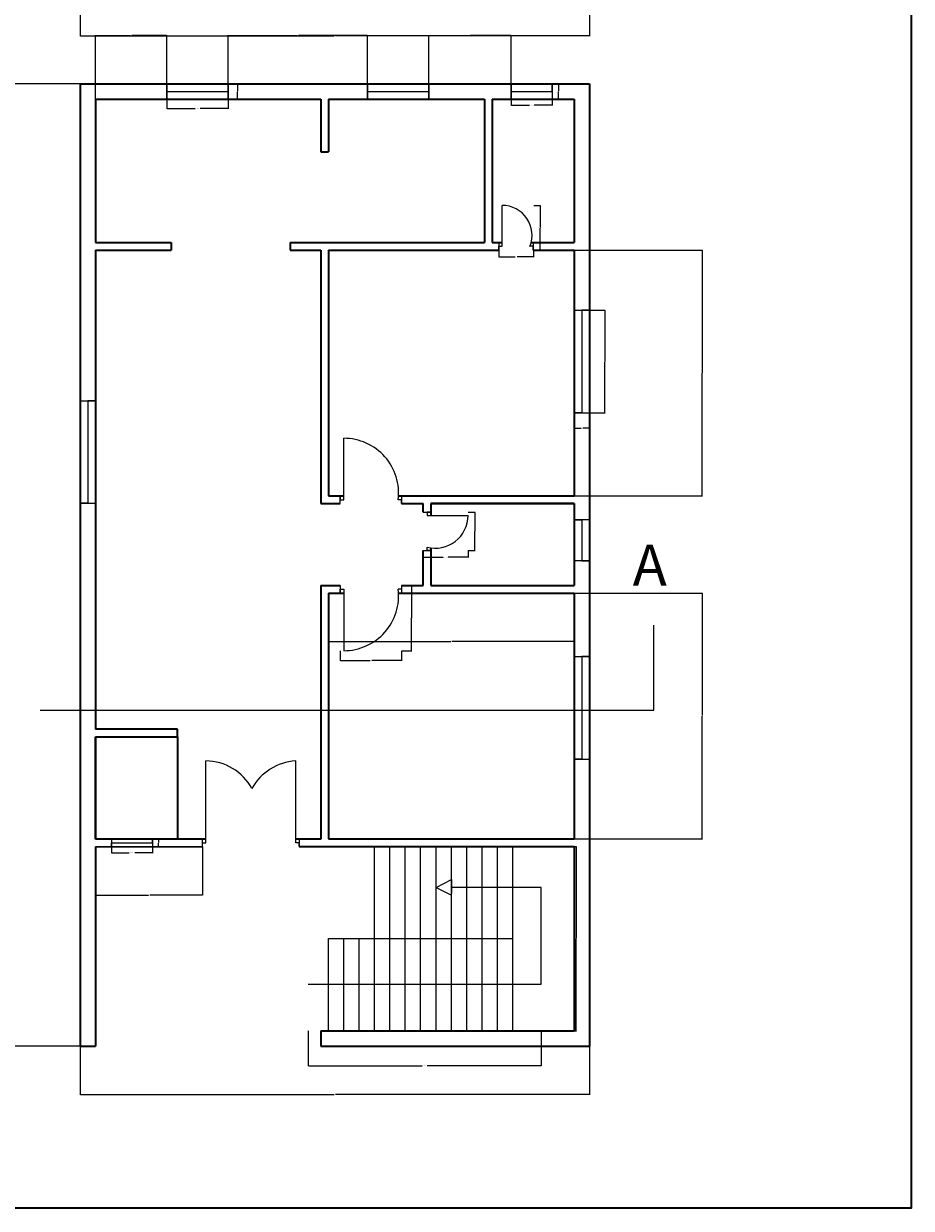
# Model space of a CAD drawing. Units: inches. Extents: x 2416 to 3391, y 1375 to 2496.
# Tile 3 of 13: x 2871 to 3391, y 1375 to 2069. Entities that reach past the tile are written whole.
import ezdxf

# ---------------------------------------------------------------- set-up
doc = ezdxf.new("R2010")
doc.units = ezdxf.units.IN
for name, color, linetype, lineweight in [('A-ANNO-DIMS', 2, 'Continuous', 18), ('A-ANNO-SYMB', 2, 'Continuous', 25), ('A-ANNO-TTLB', 7, 'Continuous', 35), ('A-DOOR', 3, 'Continuous', 20), ('A-FLOR-STRS', 7, 'Continuous', 20), ('A-GLAZ', 4, 'Continuous', 18), ('A-WALL', 7, 'Continuous', 35)]:
    doc.layers.add(name, color=color, linetype=linetype, lineweight=lineweight)
doc.styles.get("Standard").update_dxf_attribs({"font": 'arial.ttf'})
doc.dimstyles.get("Standard").update_dxf_attribs({"dimtxt": 0.18, "dimasz": 0.18, "dimexe": 0.18, "dimexo": 0.0625, "dimgap": 0.09, "dimtad": 0, "dimtih": 1, "dimtoh": 1, "dimdec": 4, "dimzin": 0, "dimdsep": 46, "dimtxsty": 'Standard', "dimcen": 0.09, "dimadec": 0, "dimazin": 0, "dimtfac": 1, "dimtdec": 4, "dimtofl": 0, "dimtmove": 0, "dimatfit": 3, "dimfxl": 1, "dimtolj": 1, "dimtzin": 0, "dimarcsym": 0})

# ---------------------------------------------------------------- blocks, each defined once
blk = doc.blocks.new('WINDOW-60IN')
for p, q in [((0, 60), (9, 60)), ((9, 60), (4.5, 60)), ((4.5, 60), (4.5, 0)), ((4.5, 0), (0, 0)), ((0, 0), (9, 0))]:
    blk.add_line(p, q)
blk = doc.blocks.new('WINDOW-36IN')
for p, q in [((0, 9), (0, 0)), ((36, 4.5), (36, 9)), ((36, 9), (36, 0)), ((0, 0), (0, 4.5)), ((0, 4.5), (36, 4.5))]:
    blk.add_line(p, q)
blk = doc.blocks.new('WINDOW-24IN')
for p, q in [((0, 9), (0, 0)), ((24, 4.5), (24, 9)), ((24, 9), (24, 0)), ((0, 0), (0, 4.5)), ((0, 4.5), (24, 4.5))]:
    blk.add_line(p, q)
blk = doc.blocks.new('WINDOW-24IN-INT')
for p, q in [((0, 4.49), (0.01, 0)), ((0.01, 0), (0, 2.24)), ((0, 2.24), (24, 2.24)), ((24, 2.24), (24, 4.49)), ((24, 4.49), (24.01, 0.03))]:
    blk.add_line(p, q)
blk = doc.blocks.new('DOOR-WC-NORTH')
for p, q in [((0, 0), (0, 24)), ((-2, 2.25), (-2, -2.25)), ((18.23, 2.25), (18.23, -2.25)), ((-2, -2.25), (-2, 0)), ((-2, 0), (0, 0)), ((18.23, 0), (16.23, 0)), ((18.23, -2.25), (18.23, 0))]:
    blk.add_line(p, q)
blk.add_arc((0, 6.51), 17.49, 338.1246, 90)
blk = doc.blocks.new('DOOR-BED-NORTH')
for p, q in [((0, 0), (0, 36)), ((-2, -2.25), (-2, 2.25)), ((-2, 2.25), (-2, 0)), ((33.94, 2.25), (33.94, -2.25)), ((-2, 0), (0, 0)), ((33.94, 0), (31.94, 0)), ((33.94, -2.25), (33.94, 0))]:
    blk.add_line(p, q)
blk.add_arc((0, 3.83), 32.17, 353.16573, 90)
blk = doc.blocks.new('DOOR-BED-SOUTH')
for p, q in [((-2, 2.25), (-2, -2.25)), ((33.94, 2.25), (33.94, -2.25)), ((-2, -2.25), (-2, 0)), ((-2, 0), (0, 0)), ((0, 0), (0, -36)), ((33.94, 0), (31.94, 0))]:
    blk.add_line(p, q)
blk.add_arc((0, -3.83), 32.17, 270, 6.83427)
blk = doc.blocks.new('DOOR-WC-SOUTH')
for p, q in [((-2.25, 2), (2.25, 2)), ((2.25, 2), (0, 2)), ((0, 2), (0, 0)), ((0, 0), (24, 0)), ((-2.25, -20.51), (2.25, -20.51)), ((0, -20.51), (0, -18.51)), ((2.25, -20.51), (0, -20.51))]:
    blk.add_line(p, q)
blk.add_arc((4.87, 0), 19.13, 255.26865, 0)
blk = doc.blocks.new('DOOR-ENTRY-PAIR')
for p, q in [((0, 0), (0, 48)), ((52.72, 0.04), (52.72, 48.04)), ((-2, 2.21), (-2, -2.21)), ((-2, 0), (0, 0)), ((54.72, 0.04), (52.72, 0.04)), ((54.72, 2.21), (54.73, -2.13)), ((54.73, -2.13), (54.72, 0.04))]:
    blk.add_line(p, q)
for centre, radius, start, end in [((0, 17.33), 30.67, 28.12018, 90), ((54.61, 16.65), 31.45, 93.43737, 151.22494)]:
    blk.add_arc(centre, radius, start, end)
blk = doc.blocks.new('STAIR-RETURN-PLAN')
for p, q in [((27, 0), (27, 108)), ((36, 0), (36, 108)), ((45, 0), (45, 108)), ((54, 0), (54, 108)), ((63, 0), (63, 108)), ((72, 0), (72, 108)), ((81, 0), (81, 108)), ((90, 0), (90, 108)), ((99, 0), (99, 108)), ((108, 0), (108, 108)), ((63, 83.93), (72, 88.71)), ((63, 83.93), (72, 79.53)), ((72, 88.71), (72, 80.54)), ((124.59, 83.93), (72, 83.93)), ((124.59, 27.37), (124.59, 83.93)), ((0, 0), (0, 54)), ((0, 54), (108, 54)), ((9, 0), (9, 54)), ((18, 0), (18, 54)), ((-11.89, 27.37), (124.59, 27.37)), ((-4.5, 0), (0, 0))]:
    blk.add_line(p, q)
blk = doc.blocks.new('*D17')
at = {"layer": 'A-ANNO-DIMS', "color": 0, "lineweight": -2, "transparency": 16777216}
for p, q in [((3202.75, 1901.41), (3211.87, 1901.41)), ((3211.69, 1901.23), (3211.69, 1871.59)), ((3211.69, 1841.59), (3211.69, 1871.23)), ((3202.75, 1841.41), (3211.87, 1841.41))]:
    blk.add_line(p, q, dxfattribs=at)
at = {"layer": 'A-ANNO-DIMS', "color": 0, "transparency": 16777216}
for points in [[(3211.66, 1901.23), (3211.72, 1901.23), (3211.69, 1901.41)], [(3211.66, 1841.59), (3211.72, 1841.59), (3211.69, 1841.41)]]:
    blk.add_solid(points, dxfattribs=at)
at = {"layer": 'Defpoints', "color": 0, "transparency": 16777216}
for p in [(3202.69, 1901.41), (3211.69, 1901.41), (3202.69, 1841.41)]:
    blk.add_point(p, dxfattribs=at)
at = {"layer": 'A-ANNO-DIMS', "color": 0, "transparency": 16777216, "insert": (3211.69, 1871.41), "char_height": 0.18, "attachment_point": 5}
blk.add_mtext('\\A1;SIDE WINDOW 60 TYP.', dxfattribs=at)
blk = doc.blocks.new('*D18')
at = {"layer": 'A-ANNO-DIMS', "color": 0, "lineweight": -2, "transparency": 16777216}
for p, q in [((3193.69, 1841.35), (3193.69, 1832.23)), ((3202.69, 1841.35), (3202.69, 1832.23)), ((3193.87, 1832.41), (3197.73, 1832.41)), ((3202.51, 1832.41), (3198.65, 1832.41))]:
    blk.add_line(p, q, dxfattribs=at)
at = {"layer": 'A-ANNO-DIMS', "color": 0, "transparency": 16777216}
for points in [[(3193.87, 1832.44), (3193.87, 1832.38), (3193.69, 1832.41)], [(3202.51, 1832.44), (3202.51, 1832.38), (3202.69, 1832.41)]]:
    blk.add_solid(points, dxfattribs=at)
at = {"layer": 'Defpoints', "color": 0, "transparency": 16777216}
for p in [(3193.69, 1841.41), (3202.69, 1841.41), (3202.69, 1832.41)]:
    blk.add_point(p, dxfattribs=at)
at = {"layer": 'A-ANNO-DIMS', "color": 0, "transparency": 16777216, "insert": (3198.19, 1832.41), "char_height": 0.18, "attachment_point": 5}
blk.add_mtext('\\A1;9 TYP.', dxfattribs=at)
blk = doc.blocks.new('*D19')
at = {"layer": 'A-ANNO-DIMS', "color": 0, "lineweight": -2, "transparency": 16777216}
for p, q in [((2954.98, 2025.11), (2954.98, 2019.59)), ((2990.98, 2025.11), (2990.98, 2019.59)), ((2955.16, 2019.77), (2971.49, 2019.77)), ((2990.8, 2019.77), (2974.48, 2019.77))]:
    blk.add_line(p, q, dxfattribs=at)
at = {"layer": 'A-ANNO-DIMS', "color": 0, "transparency": 16777216}
for points in [[(2955.16, 2019.8), (2955.16, 2019.74), (2954.98, 2019.77)], [(2990.8, 2019.8), (2990.8, 2019.74), (2990.98, 2019.77)]]:
    blk.add_solid(points, dxfattribs=at)
at = {"layer": 'Defpoints', "color": 0, "transparency": 16777216}
for p in [(2954.98, 2025.17), (2990.98, 2025.17), (2990.98, 2019.77)]:
    blk.add_point(p, dxfattribs=at)
at = {"layer": 'A-ANNO-DIMS', "color": 0, "transparency": 16777216, "insert": (2972.98, 2019.77), "char_height": 0.18, "attachment_point": 5}
blk.add_mtext('\\A1;REAR WINDOW 36 TYP.', dxfattribs=at)
blk = doc.blocks.new('*D20')
at = {"layer": 'A-ANNO-DIMS', "color": 0, "lineweight": -2, "transparency": 16777216}
for p, q in [((2991.04, 2034.17), (2996.56, 2034.17)), ((2996.38, 2033.99), (2996.38, 2029.85)), ((2996.38, 2025.35), (2996.38, 2029.49)), ((2991.04, 2025.17), (2996.56, 2025.17))]:
    blk.add_line(p, q, dxfattribs=at)
at = {"layer": 'A-ANNO-DIMS', "color": 0, "transparency": 16777216}
for points in [[(2996.35, 2033.99), (2996.41, 2033.99), (2996.38, 2034.17)], [(2996.35, 2025.35), (2996.41, 2025.35), (2996.38, 2025.17)]]:
    blk.add_solid(points, dxfattribs=at)
at = {"layer": 'Defpoints', "color": 0, "transparency": 16777216}
for p in [(2990.98, 2034.17), (2996.38, 2034.17), (2990.98, 2025.17)]:
    blk.add_point(p, dxfattribs=at)
at = {"layer": 'A-ANNO-DIMS', "color": 0, "transparency": 16777216, "insert": (2996.38, 2029.67), "char_height": 0.18, "attachment_point": 5}
blk.add_mtext('\\A1;9 TYP.', dxfattribs=at)
blk = doc.blocks.new('*D21')
at = {"layer": 'A-ANNO-DIMS', "color": 0, "lineweight": -2, "transparency": 16777216}
for p, q in [((3156.77, 2025.11), (3156.77, 2021.39)), ((3156.95, 2021.57), (3167.4, 2021.57)), ((3180.59, 2021.57), (3170.13, 2021.57)), ((3180.77, 2025.11), (3180.77, 2021.39))]:
    blk.add_line(p, q, dxfattribs=at)
at = {"layer": 'A-ANNO-DIMS', "color": 0, "transparency": 16777216}
for points in [[(3156.95, 2021.6), (3156.95, 2021.54), (3156.77, 2021.57)], [(3180.59, 2021.6), (3180.59, 2021.54), (3180.77, 2021.57)]]:
    blk.add_solid(points, dxfattribs=at)
at = {"layer": 'Defpoints', "color": 0, "transparency": 16777216}
for p in [(3156.77, 2025.17), (3180.77, 2025.17), (3180.77, 2021.57)]:
    blk.add_point(p, dxfattribs=at)
at = {"layer": 'A-ANNO-DIMS', "color": 0, "transparency": 16777216, "insert": (3168.77, 2021.57), "char_height": 0.18, "attachment_point": 5}
blk.add_mtext('\\A1;WC WINDOW 24 TYP.', dxfattribs=at)
blk = doc.blocks.new('*D22')
at = {"layer": 'A-ANNO-DIMS', "color": 0, "lineweight": -2, "transparency": 16777216}
for p, q in [((3180.83, 2034.17), (3184.55, 2034.17)), ((3184.37, 2033.99), (3184.37, 2029.85)), ((3184.37, 2025.35), (3184.37, 2029.49)), ((3180.83, 2025.17), (3184.55, 2025.17))]:
    blk.add_line(p, q, dxfattribs=at)
at = {"layer": 'A-ANNO-DIMS', "color": 0, "transparency": 16777216}
for points in [[(3184.34, 2033.99), (3184.4, 2033.99), (3184.37, 2034.17)], [(3184.34, 2025.35), (3184.4, 2025.35), (3184.37, 2025.17)]]:
    blk.add_solid(points, dxfattribs=at)
at = {"layer": 'Defpoints', "color": 0, "transparency": 16777216}
for p in [(3180.77, 2034.17), (3184.37, 2034.17), (3180.77, 2025.17)]:
    blk.add_point(p, dxfattribs=at)
at = {"layer": 'A-ANNO-DIMS', "color": 0, "transparency": 16777216, "insert": (3184.37, 2029.67), "char_height": 0.18, "attachment_point": 5}
blk.add_mtext('\\A1;9 TYP.', dxfattribs=at)
blk = doc.blocks.new('*D23')
at = {"layer": 'A-ANNO-DIMS', "color": 0, "lineweight": -2, "transparency": 16777216}
for p, q in [((2922.56, 1586.94), (2922.56, 1583.22)), ((2922.74, 1583.4), (2932.97, 1583.4)), ((2946.39, 1583.4), (2936.17, 1583.4)), ((2946.57, 1586.94), (2946.57, 1583.22))]:
    blk.add_line(p, q, dxfattribs=at)
at = {"layer": 'A-ANNO-DIMS', "color": 0, "transparency": 16777216}
for points in [[(2922.74, 1583.43), (2922.74, 1583.37), (2922.56, 1583.4)], [(2946.39, 1583.43), (2946.39, 1583.37), (2946.57, 1583.4)]]:
    blk.add_solid(points, dxfattribs=at)
at = {"layer": 'Defpoints', "color": 0, "transparency": 16777216}
for p in [(2922.56, 1587), (2946.57, 1587), (2946.57, 1583.4)]:
    blk.add_point(p, dxfattribs=at)
at = {"layer": 'A-ANNO-DIMS', "color": 0, "transparency": 16777216, "insert": (2934.57, 1583.4), "char_height": 0.18, "attachment_point": 5}
blk.add_mtext('\\A1;PORCH WINDOW 24 TYP.', dxfattribs=at)
blk = doc.blocks.new('*D24')
at = {"layer": 'A-ANNO-DIMS', "color": 0, "lineweight": -2, "transparency": 16777216}
for p, q in [((2946.63, 1591.49), (2950.35, 1591.49)), ((2950.17, 1591.31), (2950.17, 1589.43)), ((2946.63, 1587), (2950.35, 1587)), ((2950.17, 1587.18), (2950.17, 1589.07))]:
    blk.add_line(p, q, dxfattribs=at)
at = {"layer": 'A-ANNO-DIMS', "color": 0, "transparency": 16777216}
for points in [[(2950.14, 1591.31), (2950.2, 1591.31), (2950.17, 1591.49)], [(2950.14, 1587.18), (2950.2, 1587.18), (2950.17, 1587)]]:
    blk.add_solid(points, dxfattribs=at)
at = {"layer": 'Defpoints', "color": 0, "transparency": 16777216}
for p in [(2946.57, 1591.49), (2950.17, 1591.49), (2946.57, 1587)]:
    blk.add_point(p, dxfattribs=at)
at = {"layer": 'A-ANNO-DIMS', "color": 0, "transparency": 16777216, "insert": (2950.17, 1589.25), "char_height": 0.18, "attachment_point": 5}
blk.add_mtext('\\A1;4 TYP.', dxfattribs=at)
blk = doc.blocks.new('*D27')
at = {"layer": 'A-ANNO-DIMS', "color": 0, "lineweight": -2, "transparency": 16777216}
for p, q in [((3169.92, 1962.92), (3173.97, 1962.92)), ((3173.79, 1962.74), (3173.79, 1949.98)), ((3173.79, 1936.85), (3173.79, 1949.61)), ((3169.92, 1936.67), (3173.97, 1936.67))]:
    blk.add_line(p, q, dxfattribs=at)
at = {"layer": 'A-ANNO-DIMS', "color": 0, "transparency": 16777216}
for points in [[(3173.76, 1962.74), (3173.82, 1962.74), (3173.79, 1962.92)], [(3173.76, 1936.85), (3173.82, 1936.85), (3173.79, 1936.67)]]:
    blk.add_solid(points, dxfattribs=at)
at = {"layer": 'Defpoints', "color": 0, "transparency": 16777216}
for p in [(3169.86, 1962.92), (3173.79, 1962.92), (3169.86, 1936.67)]:
    blk.add_point(p, dxfattribs=at)
at = {"layer": 'A-ANNO-DIMS', "color": 0, "transparency": 16777216, "insert": (3173.79, 1949.8), "char_height": 0.18, "attachment_point": 5}
blk.add_mtext('\\A1;REAR WC DOOR 26 TYP.', dxfattribs=at)
blk = doc.blocks.new('*D28')
at = {"layer": 'A-ANNO-DIMS', "color": 0, "lineweight": -2, "transparency": 16777216}
for p, q in [((3149.47, 1936.61), (3149.47, 1932.55)), ((3149.65, 1932.73), (3159.13, 1932.73)), ((3169.68, 1932.73), (3160.19, 1932.73)), ((3169.86, 1936.61), (3169.86, 1932.55))]:
    blk.add_line(p, q, dxfattribs=at)
at = {"layer": 'A-ANNO-DIMS', "color": 0, "transparency": 16777216}
for points in [[(3149.65, 1932.76), (3149.65, 1932.7), (3149.47, 1932.73)], [(3169.68, 1932.76), (3169.68, 1932.7), (3169.86, 1932.73)]]:
    blk.add_solid(points, dxfattribs=at)
at = {"layer": 'Defpoints', "color": 0, "transparency": 16777216}
for p in [(3149.47, 1936.67), (3169.86, 1936.67), (3169.86, 1932.73)]:
    blk.add_point(p, dxfattribs=at)
at = {"layer": 'A-ANNO-DIMS', "color": 0, "transparency": 16777216, "insert": (3159.66, 1932.73), "char_height": 0.18, "attachment_point": 5}
blk.add_mtext('\\A1;20 TYP.', dxfattribs=at)
blk = doc.blocks.new('*D29')
at = {"layer": 'A-ANNO-DIMS', "color": 0, "lineweight": -2, "transparency": 16777216}
for p, q in [((3105.19, 1760.57), (3105.19, 1756.51)), ((3105.37, 1756.69), (3116.79, 1756.69)), ((3131.26, 1756.69), (3119.85, 1756.69)), ((3131.44, 1760.57), (3131.44, 1756.51))]:
    blk.add_line(p, q, dxfattribs=at)
at = {"layer": 'A-ANNO-DIMS', "color": 0, "transparency": 16777216}
for points in [[(3105.37, 1756.72), (3105.37, 1756.66), (3105.19, 1756.69)], [(3131.26, 1756.72), (3131.26, 1756.66), (3131.44, 1756.69)]]:
    blk.add_solid(points, dxfattribs=at)
at = {"layer": 'Defpoints', "color": 0, "transparency": 16777216}
for p in [(3105.19, 1760.63), (3131.44, 1760.63), (3131.44, 1756.69)]:
    blk.add_point(p, dxfattribs=at)
at = {"layer": 'A-ANNO-DIMS', "color": 0, "transparency": 16777216, "insert": (3118.32, 1756.69), "char_height": 0.18, "attachment_point": 5}
blk.add_mtext('\\A1;HALL WC DOOR 26 TYP.', dxfattribs=at)
blk = doc.blocks.new('*D30')
at = {"layer": 'A-ANNO-DIMS', "color": 0, "lineweight": -2, "transparency": 16777216}
for p, q in [((3131.5, 1783.13), (3135.56, 1783.13)), ((3135.38, 1782.95), (3135.38, 1772.06)), ((3135.38, 1760.81), (3135.38, 1771.7)), ((3131.5, 1760.63), (3135.56, 1760.63))]:
    blk.add_line(p, q, dxfattribs=at)
at = {"layer": 'A-ANNO-DIMS', "color": 0, "transparency": 16777216}
for points in [[(3135.35, 1782.95), (3135.41, 1782.95), (3135.38, 1783.13)], [(3135.35, 1760.81), (3135.41, 1760.81), (3135.38, 1760.63)]]:
    blk.add_solid(points, dxfattribs=at)
at = {"layer": 'Defpoints', "color": 0, "transparency": 16777216}
for p in [(3131.44, 1783.13), (3135.38, 1783.13), (3131.44, 1760.63)]:
    blk.add_point(p, dxfattribs=at)
at = {"layer": 'A-ANNO-DIMS', "color": 0, "transparency": 16777216, "insert": (3135.38, 1771.88), "char_height": 0.18, "attachment_point": 5}
blk.add_mtext('\\A1;23 TYP.', dxfattribs=at)
blk = doc.blocks.new('*D33')
at = {"layer": 'A-ANNO-DIMS', "color": 0, "lineweight": -2, "transparency": 16777216}
for p, q in [((3092.63, 1740.17), (3098.48, 1740.17)), ((3098.3, 1739.99), (3098.3, 1721.23)), ((3098.3, 1702.1), (3098.3, 1720.86)), ((3092.63, 1701.92), (3098.48, 1701.92))]:
    blk.add_line(p, q, dxfattribs=at)
at = {"layer": 'A-ANNO-DIMS', "color": 0, "transparency": 16777216}
for points in [[(3098.27, 1739.99), (3098.33, 1739.99), (3098.3, 1740.17)], [(3098.27, 1702.1), (3098.33, 1702.1), (3098.3, 1701.92)]]:
    blk.add_solid(points, dxfattribs=at)
at = {"layer": 'Defpoints', "color": 0, "transparency": 16777216}
for p in [(3092.56, 1740.17), (3098.3, 1740.17), (3092.56, 1701.92)]:
    blk.add_point(p, dxfattribs=at)
at = {"layer": 'A-ANNO-DIMS', "color": 0, "transparency": 16777216, "insert": (3098.3, 1721.05), "char_height": 0.18, "attachment_point": 5}
blk.add_mtext('\\A1;BEDROOM 1 DOOR 38 TYP.', dxfattribs=at)
blk = doc.blocks.new('*D34')
at = {"layer": 'A-ANNO-DIMS', "color": 0, "lineweight": -2, "transparency": 16777216}
for p, q in [((3056.62, 1701.86), (3056.62, 1696)), ((3092.56, 1701.86), (3092.56, 1696)), ((3056.8, 1696.18), (3074.06, 1696.18)), ((3092.38, 1696.18), (3075.12, 1696.18))]:
    blk.add_line(p, q, dxfattribs=at)
at = {"layer": 'A-ANNO-DIMS', "color": 0, "transparency": 16777216}
for points in [[(3056.8, 1696.21), (3056.8, 1696.15), (3056.62, 1696.18)], [(3092.38, 1696.21), (3092.38, 1696.15), (3092.56, 1696.18)]]:
    blk.add_solid(points, dxfattribs=at)
at = {"layer": 'Defpoints', "color": 0, "transparency": 16777216}
for p in [(3056.62, 1701.92), (3092.56, 1701.92), (3092.56, 1696.18)]:
    blk.add_point(p, dxfattribs=at)
at = {"layer": 'A-ANNO-DIMS', "color": 0, "transparency": 16777216, "insert": (3074.59, 1696.18), "char_height": 0.18, "attachment_point": 5}
blk.add_mtext('\\A1;36 TYP.', dxfattribs=at)
blk = doc.blocks.new('*D37')
at = {"layer": 'A-ANNO-DIMS', "color": 0, "lineweight": -2, "transparency": 16777216}
for p, q in [((3037.8, 1479.11), (3037.8, 1458.52)), ((3174.28, 1479.11), (3174.28, 1458.52)), ((3037.98, 1458.7), (3104.49, 1458.7)), ((3174.1, 1458.7), (3107.6, 1458.7))]:
    blk.add_line(p, q, dxfattribs=at)
at = {"layer": 'A-ANNO-DIMS', "color": 0, "transparency": 16777216}
for points in [[(3037.98, 1458.73), (3037.98, 1458.67), (3037.8, 1458.7)], [(3174.1, 1458.73), (3174.1, 1458.67), (3174.28, 1458.7)]]:
    blk.add_solid(points, dxfattribs=at)
at = {"layer": 'Defpoints', "color": 0, "transparency": 16777216}
for p in [(3037.8, 1479.17), (3174.28, 1479.17), (3174.28, 1458.7)]:
    blk.add_point(p, dxfattribs=at)
at = {"layer": 'A-ANNO-DIMS', "color": 0, "transparency": 16777216, "insert": (3106.04, 1458.7), "char_height": 0.18, "attachment_point": 5}
blk.add_mtext('\\A1;RETURN STAIR 136 TYP.', dxfattribs=at)
blk = doc.blocks.new('*D38')
at = {"layer": 'A-ANNO-DIMS', "color": 0, "lineweight": -2, "transparency": 16777216}
for p, q in [((3174.35, 1587.17), (3194.93, 1587.17)), ((3194.75, 1586.99), (3194.75, 1533.35)), ((3194.75, 1479.35), (3194.75, 1532.99)), ((3174.35, 1479.17), (3194.93, 1479.17))]:
    blk.add_line(p, q, dxfattribs=at)
at = {"layer": 'A-ANNO-DIMS', "color": 0, "transparency": 16777216}
for points in [[(3194.72, 1586.99), (3194.78, 1586.99), (3194.75, 1587.17)], [(3194.72, 1479.35), (3194.78, 1479.35), (3194.75, 1479.17)]]:
    blk.add_solid(points, dxfattribs=at)
at = {"layer": 'Defpoints', "color": 0, "transparency": 16777216}
for p in [(3174.28, 1587.17), (3194.75, 1587.17), (3174.28, 1479.17)]:
    blk.add_point(p, dxfattribs=at)
at = {"layer": 'A-ANNO-DIMS', "color": 0, "transparency": 16777216, "insert": (3194.75, 1533.17), "char_height": 0.18, "attachment_point": 5}
blk.add_mtext('\\A1;108 TYP.', dxfattribs=at)
blk = doc.blocks.new('*D54')
at = {"layer": 'A-ANNO-DIMS', "color": 0, "lineweight": -2, "transparency": 16777216}
for p, q in [((2904.19, 1470.11), (2904.19, 1441.64)), ((3202.69, 1470.11), (3202.69, 1441.64)), ((2904.37, 1441.82), (3053.05, 1441.82)), ((3202.51, 1441.82), (3053.84, 1441.82))]:
    blk.add_line(p, q, dxfattribs=at)
at = {"layer": 'A-ANNO-DIMS', "color": 0, "transparency": 16777216}
for points in [[(2904.37, 1441.85), (2904.37, 1441.79), (2904.19, 1441.82)], [(3202.51, 1441.85), (3202.51, 1441.79), (3202.69, 1441.82)]]:
    blk.add_solid(points, dxfattribs=at)
at = {"layer": 'Defpoints', "color": 0, "transparency": 16777216}
for p in [(2904.19, 1470.17), (3202.69, 1470.17), (3202.69, 1441.82)]:
    blk.add_point(p, dxfattribs=at)
at = {"layer": 'A-ANNO-DIMS', "color": 0, "transparency": 16777216, "insert": (3053.44, 1441.82), "char_height": 0.18, "attachment_point": 5}
blk.add_mtext('\\A1;298.5', dxfattribs=at)
blk = doc.blocks.new('*D55')
at = {"layer": 'A-ANNO-DIMS', "color": 0, "lineweight": -2, "transparency": 16777216}
for p, q in [((2904.13, 2034.17), (2852.3, 2034.17)), ((2852.48, 2033.99), (2852.48, 1752.35)), ((2852.48, 1470.35), (2852.48, 1751.99)), ((2904.13, 1470.17), (2852.3, 1470.17))]:
    blk.add_line(p, q, dxfattribs=at)
at = {"layer": 'A-ANNO-DIMS', "color": 0, "transparency": 16777216}
for points in [[(2852.45, 2033.99), (2852.51, 2033.99), (2852.48, 2034.17)], [(2852.45, 1470.35), (2852.51, 1470.35), (2852.48, 1470.17)]]:
    blk.add_solid(points, dxfattribs=at)
at = {"layer": 'Defpoints', "color": 0, "transparency": 16777216}
for p in [(2852.48, 2034.17), (2904.19, 2034.17), (2904.19, 1470.17)]:
    blk.add_point(p, dxfattribs=at)
at = {"layer": 'A-ANNO-DIMS', "color": 0, "transparency": 16777216, "insert": (2852.48, 1752.17), "char_height": 0.18, "attachment_point": 5}
blk.add_mtext('\\A1;564', dxfattribs=at)
blk = doc.blocks.new('*D56')
at = {"layer": 'A-ANNO-DIMS', "color": 0, "lineweight": -2, "transparency": 16777216}
for p, q in [((2913.19, 2025.23), (2913.19, 2062.7)), ((2913.37, 2062.52), (2933.69, 2062.52)), ((2954.8, 2062.52), (2934.48, 2062.52)), ((2954.98, 2025.23), (2954.98, 2062.7))]:
    blk.add_line(p, q, dxfattribs=at)
at = {"layer": 'A-ANNO-DIMS', "color": 0, "transparency": 16777216}
for points in [[(2913.37, 2062.55), (2913.37, 2062.49), (2913.19, 2062.52)], [(2954.8, 2062.55), (2954.8, 2062.49), (2954.98, 2062.52)]]:
    blk.add_solid(points, dxfattribs=at)
at = {"layer": 'Defpoints', "color": 0, "transparency": 16777216}
for p in [(2954.98, 2062.52), (2913.19, 2025.17), (2954.98, 2025.17)]:
    blk.add_point(p, dxfattribs=at)
at = {"layer": 'A-ANNO-DIMS', "color": 0, "transparency": 16777216, "insert": (2934.09, 2062.52), "char_height": 0.18, "attachment_point": 5}
blk.add_mtext('\\A1;41.79', dxfattribs=at)
blk = doc.blocks.new('*D57')
at = {"layer": 'A-ANNO-DIMS', "color": 0, "lineweight": -2, "transparency": 16777216}
for p, q in [((2990.98, 2025.23), (2990.98, 2062.7)), ((2991.16, 2062.52), (3031.33, 2062.52)), ((3072.29, 2062.52), (3032.12, 2062.52)), ((3072.47, 2025.23), (3072.47, 2062.7))]:
    blk.add_line(p, q, dxfattribs=at)
at = {"layer": 'A-ANNO-DIMS', "color": 0, "transparency": 16777216}
for points in [[(2991.16, 2062.55), (2991.16, 2062.49), (2990.98, 2062.52)], [(3072.29, 2062.55), (3072.29, 2062.49), (3072.47, 2062.52)]]:
    blk.add_solid(points, dxfattribs=at)
at = {"layer": 'Defpoints', "color": 0, "transparency": 16777216}
for p in [(3072.47, 2062.52), (2990.98, 2025.17), (3072.47, 2025.17)]:
    blk.add_point(p, dxfattribs=at)
at = {"layer": 'A-ANNO-DIMS', "color": 0, "transparency": 16777216, "insert": (3031.72, 2062.52), "char_height": 0.18, "attachment_point": 5}
blk.add_mtext('\\A1;81.48', dxfattribs=at)
blk = doc.blocks.new('*D58')
at = {"layer": 'A-ANNO-DIMS', "color": 0, "lineweight": -2, "transparency": 16777216}
for p, q in [((3108.47, 2025.23), (3108.47, 2062.7)), ((3108.65, 2062.52), (3132.29, 2062.52)), ((3156.59, 2062.52), (3132.94, 2062.52)), ((3156.77, 2025.23), (3156.77, 2062.7))]:
    blk.add_line(p, q, dxfattribs=at)
at = {"layer": 'A-ANNO-DIMS', "color": 0, "transparency": 16777216}
for points in [[(3108.65, 2062.55), (3108.65, 2062.49), (3108.47, 2062.52)], [(3156.59, 2062.55), (3156.59, 2062.49), (3156.77, 2062.52)]]:
    blk.add_solid(points, dxfattribs=at)
at = {"layer": 'Defpoints', "color": 0, "transparency": 16777216}
for p in [(3156.77, 2062.52), (3108.47, 2025.17), (3156.77, 2025.17)]:
    blk.add_point(p, dxfattribs=at)
at = {"layer": 'A-ANNO-DIMS', "color": 0, "transparency": 16777216, "insert": (3132.62, 2062.52), "char_height": 0.18, "attachment_point": 5}
blk.add_mtext('\\A1;48.3', dxfattribs=at)
blk = doc.blocks.new('*D59')
at = {"layer": 'A-ANNO-DIMS', "color": 0, "lineweight": -2, "transparency": 16777216}
for p, q in [((3049.69, 1735.61), (3049.69, 1707.14)), ((3193.69, 1735.61), (3193.69, 1707.14)), ((3049.87, 1707.32), (3121.41, 1707.32)), ((3193.51, 1707.32), (3121.97, 1707.32))]:
    blk.add_line(p, q, dxfattribs=at)
at = {"layer": 'A-ANNO-DIMS', "color": 0, "transparency": 16777216}
for points in [[(3049.87, 1707.35), (3049.87, 1707.29), (3049.69, 1707.32)], [(3193.51, 1707.35), (3193.51, 1707.29), (3193.69, 1707.32)]]:
    blk.add_solid(points, dxfattribs=at)
at = {"layer": 'Defpoints', "color": 0, "transparency": 16777216}
for p in [(3049.69, 1735.67), (3193.69, 1735.67), (3049.69, 1707.32)]:
    blk.add_point(p, dxfattribs=at)
at = {"layer": 'A-ANNO-DIMS', "color": 0, "transparency": 16777216, "insert": (3121.69, 1707.32), "char_height": 0.18, "attachment_point": 5}
blk.add_mtext('\\A1;144', dxfattribs=at)
blk = doc.blocks.new('*D60')
at = {"layer": 'A-ANNO-DIMS', "color": 0, "lineweight": -2, "transparency": 16777216}
for p, q in [((3193.75, 1936.67), (3268.85, 1936.67)), ((3268.67, 1936.49), (3268.67, 1864.85)), ((3268.67, 1792.85), (3268.67, 1864.49)), ((3193.75, 1792.67), (3268.85, 1792.67))]:
    blk.add_line(p, q, dxfattribs=at)
at = {"layer": 'A-ANNO-DIMS', "color": 0, "transparency": 16777216}
for points in [[(3268.64, 1936.49), (3268.7, 1936.49), (3268.67, 1936.67)], [(3268.64, 1792.85), (3268.7, 1792.85), (3268.67, 1792.67)]]:
    blk.add_solid(points, dxfattribs=at)
at = {"layer": 'Defpoints', "color": 0, "transparency": 16777216}
for p in [(3193.69, 1936.67), (3268.67, 1936.67), (3193.69, 1792.67)]:
    blk.add_point(p, dxfattribs=at)
at = {"layer": 'A-ANNO-DIMS', "color": 0, "transparency": 16777216, "insert": (3268.67, 1864.67), "char_height": 0.18, "attachment_point": 5}
blk.add_mtext('\\A1;144', dxfattribs=at)
blk = doc.blocks.new('*D61')
at = {"layer": 'A-ANNO-DIMS', "color": 0, "lineweight": -2, "transparency": 16777216}
for p, q in [((3193.75, 1735.67), (3268.85, 1735.67)), ((3268.67, 1735.49), (3268.67, 1663.85)), ((3268.67, 1591.85), (3268.67, 1663.49)), ((3193.75, 1591.67), (3268.85, 1591.67))]:
    blk.add_line(p, q, dxfattribs=at)
at = {"layer": 'A-ANNO-DIMS', "color": 0, "transparency": 16777216}
for points in [[(3268.64, 1735.49), (3268.7, 1735.49), (3268.67, 1735.67)], [(3268.64, 1591.85), (3268.7, 1591.85), (3268.67, 1591.67)]]:
    blk.add_solid(points, dxfattribs=at)
at = {"layer": 'Defpoints', "color": 0, "transparency": 16777216}
for p in [(3193.69, 1735.67), (3268.67, 1735.67), (3193.69, 1591.67)]:
    blk.add_point(p, dxfattribs=at)
at = {"layer": 'A-ANNO-DIMS', "color": 0, "transparency": 16777216, "insert": (3268.67, 1663.67), "char_height": 0.18, "attachment_point": 5}
blk.add_mtext('\\A1;144', dxfattribs=at)
blk = doc.blocks.new('*D62')
at = {"layer": 'A-ANNO-DIMS', "color": 0, "lineweight": -2, "transparency": 16777216}
for p, q in [((2913.19, 1586.93), (2913.23, 1558.46)), ((2975.76, 1587.01), (2975.8, 1558.55)), ((2913.41, 1558.64), (2944.12, 1558.68)), ((2975.62, 1558.72), (2944.91, 1558.68))]:
    blk.add_line(p, q, dxfattribs=at)
at = {"layer": 'A-ANNO-DIMS', "color": 0, "transparency": 16777216}
for points in [[(2913.41, 1558.67), (2913.41, 1558.61), (2913.23, 1558.64)], [(2975.62, 1558.75), (2975.62, 1558.69), (2975.8, 1558.73)]]:
    blk.add_solid(points, dxfattribs=at)
at = {"layer": 'Defpoints', "color": 0, "transparency": 16777216}
for p in [(2913.19, 1586.99), (2975.76, 1587.08), (2913.23, 1558.64)]:
    blk.add_point(p, dxfattribs=at)
at = {"layer": 'A-ANNO-DIMS', "color": 0, "transparency": 16777216, "insert": (2944.51, 1558.68), "char_height": 0.18, "attachment_point": 5}
blk.add_mtext('\\A1;62.57', dxfattribs=at)
blk = doc.blocks.new('*D83')
at = {"layer": 'A-ANNO-DIMS', "color": 0, "lineweight": -2, "transparency": 16777216}
for p, q in [((2904.19, 2125.8), (2904.19, 2062.03)), ((3202.69, 2125.8), (3202.69, 2062.03)), ((2904.37, 2062.21), (3053.05, 2062.21)), ((3202.51, 2062.21), (3053.84, 2062.21))]:
    blk.add_line(p, q, dxfattribs=at)
at = {"layer": 'A-ANNO-DIMS', "color": 0, "transparency": 16777216}
for points in [[(2904.37, 2062.24), (2904.37, 2062.18), (2904.19, 2062.21)], [(3202.51, 2062.24), (3202.51, 2062.18), (3202.69, 2062.21)]]:
    blk.add_solid(points, dxfattribs=at)
at = {"layer": 'Defpoints', "color": 0, "transparency": 16777216}
for p in [(2904.19, 2125.86), (3202.69, 2125.86), (3202.69, 2062.21)]:
    blk.add_point(p, dxfattribs=at)
at = {"layer": 'A-ANNO-DIMS', "color": 0, "transparency": 16777216, "insert": (3053.44, 2062.21), "char_height": 0.18, "attachment_point": 5}
blk.add_mtext('\\A1;298.5', dxfattribs=at)

msp = doc.modelspace()

# ---------------------------------------------------------------- linework, layer by layer
at = {"layer": 'A-ANNO-SYMB'}
for p, q in [((3240.3152, 1666.9855), (3240.3152, 1716.9621)), ((2880.8281, 1666.9855), (3240.3152, 1666.9855))]:
    msp.add_line(p, q, dxfattribs=at)
at = {"layer": 'A-ANNO-TTLB'}
msp.add_lwpolyline([(2416.4678, 2496.0939), (3391.2022, 2496.0939), (3391.2022, 1375.1104), (2416.4678, 1375.1104)], close=True, dxfattribs=at)
at = {"layer": 'A-WALL'}
for p, q in [((2904.1924, 2034.17), (2904.1924, 1470.17)), ((2904.1924, 2034.17), (3202.6924, 2034.17)), ((3202.6924, 2034.17), (3202.6924, 1470.17)), ((2913.1924, 2025.17), (2913.1924, 1941.17)), ((2913.1924, 2025.17), (3045.1924, 2025.17)), ((3045.1924, 2025.17), (3045.1924, 1994.3212)), ((3049.6924, 2025.17), (3049.6924, 1994.3212)), ((3049.6924, 2025.17), (3141.1924, 2025.17)), ((3141.1924, 2025.17), (3141.1924, 1941.17)), ((3145.6924, 2025.17), (3145.6924, 1941.17)), ((3145.6924, 2025.17), (3193.6924, 2025.17)), ((3193.6924, 2025.17), (3193.6924, 1941.17)), ((3045.1924, 1994.3212), (3049.6924, 1994.3212)), ((2913.1924, 1941.17), (2957.5166, 1941.17)), ((2957.5166, 1941.17), (2957.5166, 1936.67)), ((3027.1924, 1941.17), (3141.1924, 1941.17)), ((3027.1924, 1941.17), (3027.1924, 1936.67)), ((3145.6924, 1941.17), (3151.4662, 1941.17)), ((3168.4233, 1941.17), (3193.6924, 1941.17)), ((2913.1924, 1936.67), (2913.1924, 1655.9896)), ((2913.1924, 1936.67), (2957.5166, 1936.67)), ((3027.1924, 1936.67), (3045.1924, 1936.67)), ((3045.1924, 1936.67), (3045.1924, 1788.17)), ((3049.6924, 1936.67), (3049.6924, 1792.67)), ((3049.6924, 1936.67), (3149.4662, 1936.67)), ((3169.6924, 1936.67), (3193.6924, 1936.67)), ((3193.6924, 1936.67), (3193.6924, 1792.67)), ((3049.6924, 1792.67), (3058.6195, 1792.67)), ((3090.7524, 1792.67), (3193.6924, 1792.67)), ((3045.1924, 1788.17), (3056.6195, 1788.17)), ((3092.5626, 1788.17), (3105.1924, 1788.17)), ((3105.1924, 1783.1345), (3105.1924, 1788.17)), ((3109.6924, 1788.17), (3193.6924, 1788.17)), ((3193.6924, 1788.17), (3109.6924, 1788.17)), ((3109.6924, 1788.17), (3109.6924, 1781.1345)), ((3193.6924, 1788.17), (3193.6924, 1740.17)), ((3105.1924, 1740.17), (3105.1924, 1760.6291)), ((3109.6924, 1762.1797), (3109.6924, 1740.17)), ((3045.1924, 1740.17), (3045.1924, 1591.4896)), ((3045.1924, 1740.17), (3056.6195, 1740.17)), ((3092.5626, 1740.17), (3105.1924, 1740.17)), ((3109.6924, 1740.17), (3193.6924, 1740.17)), ((3049.6924, 1735.67), (3049.6924, 1591.67)), ((3049.6924, 1735.67), (3058.6195, 1735.67)), ((3090.7524, 1735.67), (3193.6924, 1735.67)), ((3193.6924, 1735.67), (3193.6924, 1591.67)), ((2961.1924, 1655.9896), (2913.1924, 1655.9896)), ((2961.1924, 1651.4896), (2961.1924, 1655.9896)), ((2913.1924, 1651.4896), (2913.1924, 1591.4896)), ((2913.1924, 1591.4896), (2913.1924, 1651.4896)), ((2913.1924, 1651.4896), (2961.1924, 1651.4896)), ((2961.1924, 1651.4896), (2961.1924, 1591.4896)), ((2977.7552, 1591.4896), (2913.1924, 1591.4896)), ((3045.1924, 1591.4896), (3030.4791, 1591.4896)), ((3049.6924, 1591.67), (3193.6924, 1591.67)), ((2913.1924, 1586.9896), (2975.7582, 1587.0751)), ((2913.1924, 1586.9896), (2913.1924, 1470.17)), ((3032.482, 1587.1527), (3045.1924, 1587.17)), ((3045.1924, 1587.17), (3193.6924, 1587.17)), ((3193.6924, 1587.17), (3193.6924, 1479.17)), ((3045.1924, 1479.17), (3045.1924, 1470.17)), ((3045.1924, 1479.17), (3193.6924, 1479.17)), ((2904.1924, 1470.17), (2913.1924, 1470.17)), ((3045.1924, 1470.17), (3202.6924, 1470.17))]:
    msp.add_line(p, q, dxfattribs=at)

# ---------------------------------------------------------------- block references
at = {"layer": 'A-DOOR'}
for name, p in [('DOOR-WC-NORTH', (3151.4662, 1938.92)), ('DOOR-BED-NORTH', (3058.6195, 1790.42)), ('DOOR-WC-SOUTH', (3107.4424, 1781.1345)), ('DOOR-BED-SOUTH', (3058.6195, 1737.92)), ('DOOR-ENTRY-PAIR', (2977.7552, 1589.2824))]:
    msp.add_blockref(name, p, dxfattribs=at)
at = {"layer": 'A-FLOR-STRS'}
msp.add_blockref('STAIR-RETURN-PLAN', (3049.6924, 1479.17), dxfattribs=at)
at = {"layer": 'A-GLAZ'}
for name, p in [('WINDOW-36IN', (2954.9821, 2025.17)), ('WINDOW-36IN', (3072.4662, 2025.17)), ('WINDOW-24IN', (3156.7671, 2025.17)), ('WINDOW-60IN', (3193.6921, 1841.41)), ('WINDOW-60IN', (2904.1921, 1788.3842)), ('WINDOW-60IN', (3193.6921, 1638.4452)), ('WINDOW-24IN-INT', (2922.5621, 1587.002))]:
    msp.add_blockref(name, p, dxfattribs=at)
at = {"layer": 'A-GLAZ', "rotation": 270.0000000000002}
msp.add_blockref('WINDOW-24IN', (3193.6924, 1778.581), dxfattribs=at)

# ---------------------------------------------------------------- texts
at = {"layer": 'A-ANNO-SYMB', "insert": (3227.9919, 1764.1232), "char_height": 24, "attachment_point": 1}
msp.add_mtext_dynamic_manual_height_columns('A', width=43.659534, gutter_width=12.5, heights=[0], dxfattribs=at)

# ---------------------------------------------------------------- dimensions: what is measured, and where the dimension line sits
at = {"layer": 'A-ANNO-DIMS'}
for base, p1, p2, override, picture, middle in [((3202.6924, 2062.2125), (2904.1924, 2125.8608), (3202.6924, 2125.8608), {"dimdec": 1, "dimlfac": 1, "dimrnd": 0, "dimzin": 0, "dimdsep": 46, "dimlunit": 2}, '*D83', (3053.4424, 2062.2125)), ((2954.9819, 2062.52), (2913.1924, 2025.17), (2954.9819, 2025.17), {"dimdec": 2, "dimlfac": 1, "dimrnd": 0, "dimzin": 0, "dimdsep": 46, "dimlunit": 2}, '*D56', (2934.0872, 2062.52)), ((3072.4661, 2062.52), (2990.9819, 2025.17), (3072.4661, 2025.17), {"dimdec": 2, "dimlfac": 1, "dimrnd": 0, "dimzin": 0, "dimdsep": 46, "dimlunit": 2}, '*D57', (3031.724, 2062.52)), ((3156.7667, 2062.52), (3108.4661, 2025.17), (3156.7667, 2025.17), {"dimdec": 1, "dimlfac": 1, "dimrnd": 0, "dimzin": 0, "dimdsep": 46, "dimlunit": 2}, '*D58', (3132.6164, 2062.52)), ((3202.6924, 1441.82), (2904.1924, 1470.17), (3202.6924, 1470.17), {"dimdec": 1, "dimlfac": 1, "dimrnd": 0, "dimzin": 0, "dimdsep": 46, "dimlunit": 2}, '*D54', (3053.4424, 1441.82))]:
    dim = msp.add_linear_dim(base=base, p1=p1, p2=p2, dimstyle='Standard', override=override, dxfattribs=at)
    dim.commit()
    dim.dimension.update_dxf_attribs({"geometry": picture, "text_midpoint": middle})
for base, p1, p2, angle, override, picture, middle in [((2852.4781, 2034.17), (2904.1924, 1470.17), (2904.1924, 2034.17), 90, {"dimdec": 0, "dimlfac": 1, "dimrnd": 0, "dimzin": 0, "dimdsep": 46, "dimlunit": 2}, '*D55', (2852.4781, 1752.17)), ((3268.6652, 1936.67), (3193.6924, 1792.67), (3193.6924, 1936.67), 90, {"dimdec": 0, "dimlfac": 1, "dimrnd": 0, "dimzin": 0, "dimdsep": 46, "dimlunit": 2}, '*D60', (3268.6652, 1864.67)), ((3049.6924, 1707.32), (3193.6924, 1735.67), (3049.6924, 1735.67), 180, {"dimdec": 0, "dimlfac": 1, "dimrnd": 0, "dimzin": 0, "dimdsep": 46, "dimlunit": 2}, '*D59', (3121.6924, 1707.32)), ((3268.6652, 1735.67), (3193.6924, 1591.67), (3193.6924, 1735.67), 90, {"dimdec": 0, "dimlfac": 1, "dimrnd": 0, "dimzin": 0, "dimdsep": 46, "dimlunit": 2}, '*D61', (3268.6652, 1663.67)), ((2913.2312, 1558.6396), (2975.7582, 1587.0751), (2913.1924, 1586.9896), 180.0783088, {"dimdec": 2, "dimlfac": 1, "dimrnd": 0, "dimzin": 0, "dimdsep": 46, "dimlunit": 2}, '*D62', (2944.514, 1558.6824))]:
    dim = msp.add_linear_dim(base=base, p1=p1, p2=p2, angle=angle, dimstyle='Standard', override=override, dxfattribs=at)
    dim.commit()
    dim.dimension.update_dxf_attribs({"geometry": picture, "text_midpoint": middle})
for base, p1, p2, text, picture, middle in [((2996.3819, 2034.17), (2990.9819, 2025.17), (2990.9819, 2034.17), '<> TYP.', '*D20', (2996.3819, 2029.67)), ((3184.3667, 2034.17), (3180.7667, 2025.17), (3180.7667, 2034.17), '<> TYP.', '*D22', (3184.3667, 2029.67)), ((3173.7932, 1962.92), (3169.8557, 1936.67), (3169.8557, 1962.92), 'REAR WC DOOR <> TYP.', '*D27', (3173.7932, 1949.795)), ((3211.6924, 1901.4103), (3202.6924, 1841.4103), (3202.6924, 1901.4103), 'SIDE WINDOW <> TYP.', '*D17', (3211.6924, 1871.4103)), ((3135.3799, 1783.1345), (3131.4424, 1760.6291), (3131.4424, 1783.1345), '<> TYP.', '*D30', (3135.3799, 1771.8818)), ((3098.3001, 1740.17), (3092.5626, 1701.92), (3092.5626, 1740.17), 'BEDROOM 1 DOOR <> TYP.', '*D33', (3098.3001, 1721.045)), ((2950.173, 1591.4896), (2946.5717, 1587.0024), (2946.5717, 1591.4896), '<> TYP.', '*D24', (2950.173, 1589.246)), ((3194.7549, 1587.17), (3174.2831, 1479.17), (3174.2831, 1587.17), '<> TYP.', '*D38', (3194.7549, 1533.17))]:
    dim = msp.add_linear_dim(base=base, p1=p1, p2=p2, angle=90, text=text, dimstyle='Standard', override={"dimdec": 0, "dimlfac": 1, "dimrnd": 0, "dimzin": 0, "dimdsep": 46, "dimlunit": 2}, dxfattribs=at)
    dim.commit()
    dim.dimension.update_dxf_attribs({"geometry": picture, "text_midpoint": middle})
for base, p1, p2, text, picture, middle in [((2990.9819, 2019.77), (2954.9819, 2025.17), (2990.9819, 2025.17), 'REAR WINDOW <> TYP.', '*D19', (2972.9819, 2019.77)), ((3180.7667, 2021.57), (3156.7667, 2025.17), (3180.7667, 2025.17), 'WC WINDOW <> TYP.', '*D21', (3168.7667, 2021.57)), ((3169.8557, 1932.7325), (3149.4662, 1936.67), (3169.8557, 1936.67), '<> TYP.', '*D28', (3159.6609, 1932.7325)), ((3202.6924, 1832.4103), (3193.6924, 1841.4103), (3202.6924, 1841.4103), '<> TYP.', '*D18', (3198.1924, 1832.4103)), ((3131.4424, 1756.6916), (3105.1924, 1760.6291), (3131.4424, 1760.6291), 'HALL WC DOOR <> TYP.', '*D29', (3118.3174, 1756.6916)), ((3092.5626, 1696.1825), (3056.6195, 1701.92), (3092.5626, 1701.92), '<> TYP.', '*D34', (3074.5911, 1696.1825)), ((2946.5717, 1583.4011), (2922.5625, 1587.0024), (2946.5717, 1587.0024), 'PORCH WINDOW <> TYP.', '*D23', (2934.5671, 1583.4011)), ((3174.2831, 1458.6982), (3037.8043, 1479.17), (3174.2831, 1479.17), 'RETURN STAIR <> TYP.', '*D37', (3106.0437, 1458.6982))]:
    dim = msp.add_linear_dim(base=base, p1=p1, p2=p2, text=text, dimstyle='Standard', override={"dimdec": 0, "dimlfac": 1, "dimrnd": 0, "dimzin": 0, "dimdsep": 46, "dimlunit": 2}, dxfattribs=at)
    dim.commit()
    dim.dimension.update_dxf_attribs({"geometry": picture, "text_midpoint": middle})

doc.saveas('drawing.dxf')
